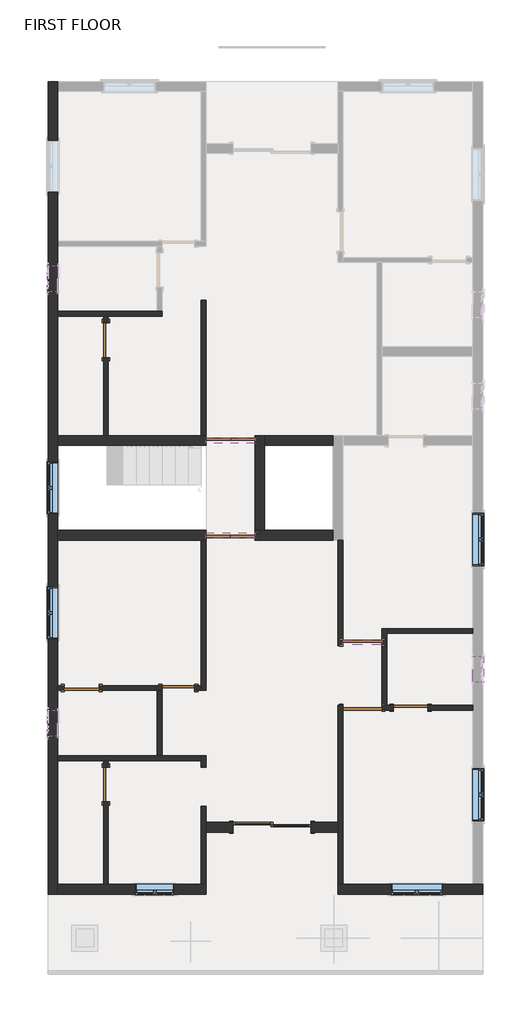
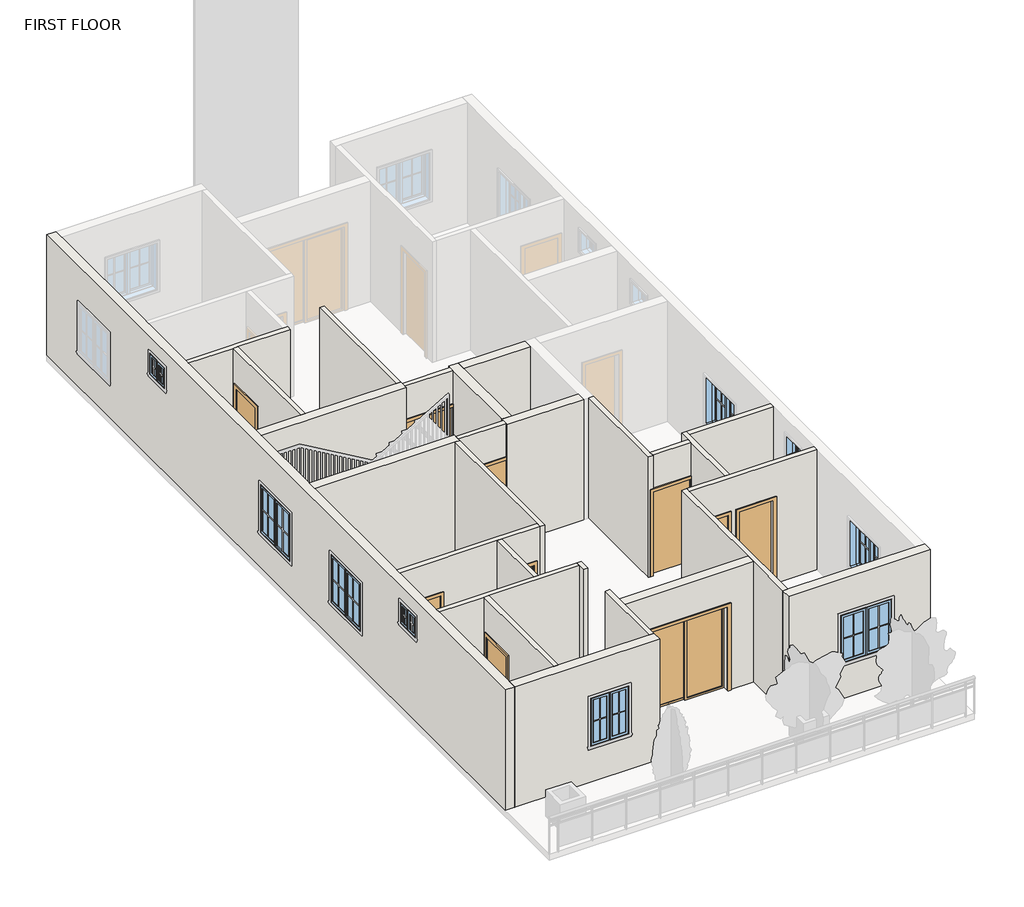
# One storey, part 1 of 4: 27 walls, 10 doors, 9 windows.
"""IFC4 building model written with IfcOpenShell, lengths in millimetres."""

from ifc_helpers import new_model, si_unit, frame, origin, place, context, project, spatial, polyline, outline, extrude, faceted_brep, transform, mapped, element, save
from components import door_31bd1cdd, door_d4d75d1e, door_214872d5, door_d141acb4, door_38851409, single_flush_3_x7_e5f9f3c4, single_flush_3_x7_305aa2a5, window_79894727, window_casement_double_3_x4_d341e8ac, window_casement_double_4_x4_af3140d2

model = new_model("IFC4")

# Units and contexts
model_context = context("Model", 3, world=origin())
ifc_project = project(units=[si_unit("LENGTHUNIT", "METRE", prefix="MILLI")], contexts=[model_context])

# Site, building, storey
site = spatial("IfcSite", under=ifc_project)
building = spatial("IfcBuilding", under=site)
storey = spatial("IfcBuildingStorey", under=building, Name="FIRST FLOOR", Elevation=3200.4)

# Doors
placement = place(None, origin())
door_shape = door_31bd1cdd(model_context)
element("IfcDoor", 1, ObjectType="Door-Double-Flush_Panel : 3'9\"X7'", at=placement, inside=storey, context=model_context, shape_type="MappedRepresentation", body=[
    mapped(door_shape, transform((-2091.0289041, 1664.1153263, 3200.4), x_axis=(1.0, 0.0, 0.0), y_axis=(0.0, 1.0, 0.0), z_axis=(0.0, 0.0, 1.0))),
])
element("IfcDoor", 2, ObjectType="Door-Double-Flush_Panel : 3'9\"X7'", at=placement, inside=storey, context=model_context, shape_type="MappedRepresentation", body=[
    mapped(door_shape, transform((-2091.0289041, -545.7007836, 3200.4), x_axis=(-1.0, 0.0, 0.0), y_axis=(0.0, -1.0, 0.0), z_axis=(0.0, 0.0, 1.0))),
])
door_2_shape = door_d4d75d1e(model_context)
element("IfcDoor", 3, ObjectType="Door-Double-Sliding : 72\" x 84\"", at=placement, inside=storey, context=model_context, shape_type="MappedRepresentation", body=[
    mapped(door_2_shape, transform((-1119.4789041, -7505.2846737, 3200.4), x_axis=(1.0, 0.0, 0.0), y_axis=(0.0, 1.0, 0.0), z_axis=(0.0, 0.0, 1.0))),
])
door_3_shape = door_214872d5(model_context)
element("IfcDoor", 4, ObjectType="Single-Flush : 2'6\"X7'", at=placement, inside=storey, context=model_context, shape_type="MappedRepresentation", body=[
    mapped(door_3_shape, transform((-3310.2289041, -4120.7346737, 3200.4), x_axis=(1.0, 0.0, 0.0), y_axis=(0.0, 1.0, 0.0), z_axis=(0.0, 0.0, 1.0))),
])
door_4_shape = door_d141acb4(model_context)
element("IfcDoor", 5, ObjectType="Single-Flush : 2'8\"X7'", at=placement, inside=storey, context=model_context, shape_type="MappedRepresentation", body=[
    mapped(door_4_shape, transform((-5005.6789041, 4013.6153263, 3200.4), x_axis=(0.0, 1.0, 0.0), y_axis=(-1.0, 0.0, 0.0), z_axis=(0.0, 0.0, 1.0))),
])
element("IfcDoor", 6, ObjectType="Single-Flush : 2'8\"X7'", at=placement, inside=storey, context=model_context, shape_type="MappedRepresentation", body=[
    mapped(door_4_shape, transform((-5570.8289041, -4120.7346737, 3200.4), x_axis=(-1.0, 0.0, 0.0), y_axis=(0.0, -1.0, 0.0), z_axis=(0.0, 0.0, 1.0))),
])
element("IfcDoor", 7, ObjectType="Single-Flush : 2'8\"X7'", at=placement, inside=storey, context=model_context, shape_type="MappedRepresentation", body=[
    mapped(door_4_shape, transform((-5005.6789041, -6374.9846737, 3200.4), x_axis=(0.0, 1.0, 0.0), y_axis=(-1.0, 0.0, 0.0), z_axis=(0.0, 0.0, 1.0))),
])
door_5_shape = door_38851409(model_context)
element("IfcDoor", 8, ObjectType="Single-Flush : 2'8\"X7'", at=placement, inside=storey, context=model_context, shape_type="MappedRepresentation", body=[
    mapped(door_5_shape, transform((2125.3710959, -4577.9346737, 3200.4), x_axis=(-1.0, 0.0, 0.0), y_axis=(0.0, -1.0, 0.0), z_axis=(0.0, 0.0, 1.0))),
])
single_flush_3_x7_shape = single_flush_3_x7_e5f9f3c4(model_context)
element("IfcDoor", 9, ObjectType="Single-Flush : 3'X7'", at=placement, inside=storey, context=model_context, shape_type="MappedRepresentation", body=[
    mapped(single_flush_3_x7_shape, transform((995.0710959, -4577.9346737, 3200.4), x_axis=(-1.0, 0.0, 0.0), y_axis=(0.0, -1.0, 0.0), z_axis=(0.0, 0.0, 1.0))),
])
single_flush_3_x7_2_shape = single_flush_3_x7_305aa2a5(model_context)
element("IfcDoor", 10, ObjectType="Single-Flush : 3'X7'", at=placement, inside=storey, context=model_context, shape_type="MappedRepresentation", body=[
    mapped(single_flush_3_x7_2_shape, transform((995.0710959, -3056.3085282, 3200.4), x_axis=(-1.0, 0.0, 0.0), y_axis=(0.0, -1.0, 0.0), z_axis=(0.0, 0.0, 1.0))),
])

# Walls
element("IfcWall", 11, ObjectType="4.5\"", at=placement, inside=storey, context=model_context, shape_type="Brep", body=[
    faceted_brep([(-6129.6289041, 4572.4153263, 3200.4), (-5062.8289041, 4572.4153263, 3200.4), (-4948.5289041, 4572.4153263, 3200.4), (-3691.2289041, 4572.4153263, 3200.4), (-3691.2289041, 4572.4153263, 6248.4), (-4948.5289041, 4572.4153263, 6248.4), (-5062.8289041, 4572.4153263, 6248.4), (-6129.6289041, 4572.4153263, 6248.4), (-6129.6289041, 4686.7153263, 3200.4), (-6129.6289041, 4686.7153263, 6248.4), (-3805.5289041, 4686.7153263, 6248.4), (-3691.2289041, 4686.7153263, 6248.4), (-3691.2289041, 4686.7153263, 3200.4), (-3805.5289041, 4686.7153263, 3200.4)], [[[0, 1, 2, 3, 4, 5, 6, 7]], [[8, 9, 10, 11, 12, 13]], [[3, 2, 1, 0, 8, 13, 12]], [[7, 6, 5, 4, 11, 10, 9]], [[0, 7, 9, 8]], [[4, 3, 12, 11]]]),
])
element("IfcWall", 12, ObjectType="4.5\"", at=placement, inside=storey, context=model_context, shape_type="SweptSolid", body=[
    extrude(outline(polyline([(4572.4153263, 3200.4), (4420.0153263, 3200.4), (4420.0153263, 5334.0), (3607.2153263, 5334.0), (3607.2153263, 3200.4), (1778.4153263, 3200.4), (1778.4153263, 6248.4), (4572.4153263, 6248.4), (4572.4153263, 3200.4)])), frame((-5062.8289041, 0.0, 0.0), z_axis=(1.0, 0.0, 0.0), x_axis=(0.0, 1.0, 0.0)), (0.0, 0.0, 1.0), 114.3),
])
element("IfcWall", 13, ObjectType="4.5\"", at=placement, inside=storey, context=model_context, shape_type="SweptSolid", body=[
    extrude(outline(polyline([(-2776.8289041, 1778.4153263), (-2776.8289041, 4948.2268555), (-2662.5289041, 4948.2268555), (-2662.5289041, 1778.4153263), (-2776.8289041, 1778.4153263)])), frame((0.0, 0.0, 3200.4), z_axis=(0.0, 0.0, 1.0), x_axis=(1.0, 0.0, 0.0)), (0.0, 0.0, 1.0), 3048.0),
])
element("IfcWall", 14, ObjectType="4.5\"", at=placement, inside=storey, context=model_context, shape_type="Brep", body=[
    faceted_brep([(-2776.8289041, -659.9846737, 3200.4), (-2776.8289041, -4063.5846737, 3200.4), (-2776.8289041, -4177.8846737, 3200.4), (-2776.8289041, -4177.8846737, 6248.4), (-2776.8289041, -4063.5846737, 6248.4), (-2776.8289041, -659.9846737, 6248.4), (-2662.5289041, -659.9846737, 3200.4), (-2662.5289041, -659.9846737, 6248.4), (-2662.5289041, -4177.8846737, 6248.4), (-2662.5289041, -4177.8846737, 3200.4)], [[[0, 1, 2, 3, 4, 5]], [[6, 7, 8, 9]], [[2, 1, 0, 6, 9]], [[5, 4, 3, 8, 7]], [[0, 5, 7, 6]], [[3, 2, 9, 8]]]),
])
element("IfcWall", 15, ObjectType="4.5\"", at=placement, inside=storey, context=model_context, shape_type="Brep", body=[
    faceted_brep([(-2776.8289041, -4063.5846737, 3200.4), (-2929.2289041, -4063.5846737, 3200.4), (-2929.2289041, -4063.5846737, 5334.0), (-3691.2289041, -4063.5846737, 5334.0), (-3691.2289041, -4063.5846737, 3200.4), (-5164.4289041, -4063.5846737, 3200.4), (-5164.4289041, -4063.5846737, 5334.0), (-5977.2289041, -4063.5846737, 5334.0), (-5977.2289041, -4063.5846737, 3200.4), (-6129.6289041, -4063.5846737, 3200.4), (-6129.6289041, -4063.5846737, 6248.4), (-2776.8289041, -4063.5846737, 6248.4), (-2929.2289041, -4177.8846737, 5334.0), (-2929.2289041, -4177.8846737, 3200.4), (-2776.8289041, -4177.8846737, 3200.4), (-2776.8289041, -4177.8846737, 6248.4), (-3691.2289041, -4177.8846737, 6248.4), (-3805.5289041, -4177.8846737, 6248.4), (-6129.6289041, -4177.8846737, 6248.4), (-6129.6289041, -4177.8846737, 3200.4), (-5977.2289041, -4177.8846737, 3200.4), (-5977.2289041, -4177.8846737, 5334.0), (-5164.4289041, -4177.8846737, 5334.0), (-5164.4289041, -4177.8846737, 3200.4), (-3805.5289041, -4177.8846737, 3200.4), (-3691.2289041, -4177.8846737, 3200.4), (-3691.2289041, -4177.8846737, 5334.0)], [[[0, 1, 2, 3, 4, 5, 6, 7, 8, 9, 10, 11]], [[12, 13, 14, 15, 16, 17, 18, 19, 20, 21, 22, 23, 24, 25, 26]], [[9, 8, 20, 19]], [[14, 13, 1, 0]], [[25, 24, 23, 5, 4]], [[11, 10, 18, 17, 16, 15]], [[0, 11, 15, 14]], [[10, 9, 19, 18]], [[21, 20, 8, 7]], [[22, 21, 7, 6]], [[23, 22, 6, 5]], [[2, 1, 13, 12]], [[3, 2, 12, 26]], [[4, 3, 26, 25]]]),
])
element("IfcWall", 16, ObjectType="4.5\"", at=placement, inside=storey, context=model_context, shape_type="Brep", body=[
    faceted_brep([(-3805.5289041, -4177.8846737, 3200.4), (-3805.5289041, -5701.8846737, 3200.4), (-3805.5289041, -5701.8846737, 6248.4), (-3805.5289041, -4177.8846737, 6248.4), (-3691.2289041, -4177.8846737, 3200.4), (-3691.2289041, -4177.8846737, 5334.0), (-3691.2289041, -4177.8846737, 6248.4), (-3691.2289041, -5701.8846737, 6248.4), (-3691.2289041, -5701.8846737, 3200.4)], [[[0, 1, 2, 3]], [[4, 5, 6, 7, 8]], [[1, 0, 4, 8]], [[3, 2, 7, 6]], [[0, 3, 6, 5, 4]], [[2, 1, 8, 7]]]),
])
element("IfcWall", 17, ObjectType="4.5\"", at=placement, inside=storey, context=model_context, shape_type="Brep", body=[
    faceted_brep([(-6129.6289041, -5816.1846737, 3200.4), (-5062.8289041, -5816.1846737, 3200.4), (-4948.5289041, -5816.1846737, 3200.4), (-2776.8289041, -5816.1846737, 3200.4), (-2776.8289041, -5816.1846737, 6248.4), (-4948.5289041, -5816.1846737, 6248.4), (-5062.8289041, -5816.1846737, 6248.4), (-6129.6289041, -5816.1846737, 6248.4), (-6129.6289041, -5701.8846737, 3200.4), (-6129.6289041, -5701.8846737, 6248.4), (-3805.5289041, -5701.8846737, 6248.4), (-3691.2289041, -5701.8846737, 6248.4), (-2776.8289041, -5701.8846737, 6248.4), (-2776.8289041, -5701.8846737, 3200.4), (-3691.2289041, -5701.8846737, 3200.4), (-3805.5289041, -5701.8846737, 3200.4)], [[[0, 1, 2, 3, 4, 5, 6, 7]], [[8, 9, 10, 11, 12, 13, 14, 15]], [[3, 2, 1, 0, 8, 15, 14, 13]], [[7, 6, 5, 4, 12, 11, 10, 9]], [[0, 7, 9, 8]], [[4, 3, 13, 12]]]),
])
element("IfcWall", 18, ObjectType="4.5\"", at=placement, inside=storey, context=model_context, shape_type="Brep", body=[
    faceted_brep([(-2776.8289041, -5701.8846737, 3200.4), (-2776.8289041, -5816.1846737, 3200.4), (-2776.8289041, -5968.5846737, 3200.4), (-2776.8289041, -5968.5846737, 6248.4), (-2776.8289041, -5816.1846737, 6248.4), (-2776.8289041, -5701.8846737, 6248.4), (-2662.5289041, -5701.8846737, 3200.4), (-2662.5289041, -5701.8846737, 6248.4), (-2662.5289041, -5968.5846737, 6248.4), (-2662.5289041, -5968.5846737, 3200.4)], [[[0, 1, 2, 3, 4, 5]], [[6, 7, 8, 9]], [[2, 1, 0, 6, 9]], [[3, 2, 9, 8]], [[5, 4, 3, 8, 7]], [[0, 5, 7, 6]]]),
])
element("IfcWall", 19, ObjectType="4.5\"", at=placement, inside=storey, context=model_context, shape_type="SweptSolid", body=[
    extrude(outline(polyline([(-5816.1846737, 3200.4), (-5968.5846737, 3200.4), (-5968.5846737, 5334.0), (-6781.3846737, 5334.0), (-6781.3846737, 3200.4), (-8711.7846737, 3200.4), (-8711.7846737, 6248.4), (-5816.1846737, 6248.4), (-5816.1846737, 3200.4)])), frame((-5062.8289041, 0.0, 0.0), z_axis=(1.0, 0.0, 0.0), x_axis=(0.0, 1.0, 0.0)), (0.0, 0.0, 1.0), 114.3),
])
element("IfcWall", 20, ObjectType="4.5\"", at=placement, inside=storey, context=model_context, shape_type="Brep", body=[
    faceted_brep([(-2776.8289041, -6882.9846737, 3200.4), (-2776.8289041, -8711.7846737, 3200.4), (-2776.8289041, -8711.7846737, 6248.4), (-2776.8289041, -6882.9846737, 6248.4), (-2662.5289041, -6882.9846737, 3200.4), (-2662.5289041, -6882.9846737, 6248.4), (-2662.5289041, -7263.9846737, 6248.4), (-2662.5289041, -7492.5846737, 6248.4), (-2662.5289041, -8711.7846737, 6248.4), (-2662.5289041, -8711.7846737, 3200.4), (-2662.5289041, -7492.5846737, 3200.4), (-2662.5289041, -7263.9846737, 3200.4)], [[[0, 1, 2, 3]], [[4, 5, 6, 7, 8, 9, 10, 11]], [[1, 0, 4, 11, 10, 9]], [[3, 2, 8, 7, 6, 5]], [[0, 3, 5, 4]], [[2, 1, 9, 8]]]),
])
element("IfcWall", 21, ObjectType="4.5\"", at=placement, inside=storey, context=model_context, shape_type="Brep", body=[
    faceted_brep([(423.5710959, -659.9846737, 3200.4), (423.5710959, -3136.3185282, 3200.4), (423.5710959, -3136.3185282, 6248.4), (423.5710959, -659.9846737, 6248.4), (537.8710959, -659.9846737, 3200.4), (537.8710959, -659.9846737, 6248.4), (537.8710959, -2999.1585282, 6248.4), (537.8710959, -3113.4585282, 6248.4), (537.8710959, -3136.3185282, 6248.4), (537.8710959, -3136.3185282, 3200.4), (537.8710959, -3113.4585282, 3200.4), (537.8710959, -2999.1585282, 3200.4)], [[[0, 1, 2, 3]], [[4, 5, 6, 7, 8, 9, 10, 11]], [[1, 0, 4, 11, 10, 9]], [[2, 1, 9, 8]], [[3, 2, 8, 7, 6, 5]], [[0, 3, 5, 4]]]),
])
element("IfcWall", 22, ObjectType="4.5\"", at=placement, inside=storey, context=model_context, shape_type="Brep", body=[
    faceted_brep([(423.5710959, -4520.7846737, 3200.4), (423.5710959, -7263.9846737, 3200.4), (423.5710959, -7492.5846737, 3200.4), (423.5710959, -8711.7846737, 3200.4), (423.5710959, -8711.7846737, 6248.4), (423.5710959, -7492.5846737, 6248.4), (423.5710959, -7263.9846737, 6248.4), (423.5710959, -4520.7846737, 6248.4), (537.8710959, -4520.7846737, 3200.4), (537.8710959, -4520.7846737, 5334.0), (537.8710959, -4520.7846737, 6248.4), (537.8710959, -4635.0846737, 6248.4), (537.8710959, -8711.7846737, 6248.4), (537.8710959, -8711.7846737, 3200.4)], [[[0, 1, 2, 3, 4, 5, 6, 7]], [[8, 9, 10, 11, 12, 13]], [[3, 2, 1, 0, 8, 13]], [[7, 6, 5, 4, 12, 11, 10]], [[4, 3, 13, 12]], [[0, 7, 10, 9, 8]]]),
])
element("IfcWall", 23, ObjectType="4.5\"", at=placement, inside=storey, context=model_context, shape_type="Brep", body=[
    faceted_brep([(1718.9710959, -4520.7846737, 5334.0), (1718.9710959, -4520.7846737, 3200.4), (1566.5710959, -4520.7846737, 3200.4), (1452.2710959, -4520.7846737, 3200.4), (1452.2710959, -4520.7846737, 5334.0), (537.8710959, -4520.7846737, 5334.0), (537.8710959, -4520.7846737, 6248.4), (1452.2710959, -4520.7846737, 6248.4), (1566.5710959, -4520.7846737, 6248.4), (3585.8710959, -4520.7846737, 6248.4), (3585.8710959, -4520.7846737, 3200.4), (2531.7710959, -4520.7846737, 3200.4), (2531.7710959, -4520.7846737, 5334.0), (1452.2710959, -4635.0846737, 3200.4), (1718.9710959, -4635.0846737, 3200.4), (1718.9710959, -4635.0846737, 5334.0), (2531.7710959, -4635.0846737, 5334.0), (2531.7710959, -4635.0846737, 3200.4), (3585.8710959, -4635.0846737, 3200.4), (3585.8710959, -4635.0846737, 6248.4), (537.8710959, -4635.0846737, 6248.4), (537.8710959, -4635.0846737, 5334.0), (1452.2710959, -4635.0846737, 5334.0)], [[[0, 1, 2, 3, 4, 5, 6, 7, 8, 9, 10, 11, 12]], [[13, 14, 15, 16, 17, 18, 19, 20, 21, 22]], [[11, 10, 18, 17]], [[3, 2, 1, 14, 13]], [[9, 8, 7, 6, 20, 19]], [[10, 9, 19, 18]], [[20, 6, 5, 21]], [[4, 22, 21, 5]], [[22, 4, 3, 13]], [[15, 14, 1, 0]], [[16, 15, 0, 12]], [[17, 16, 12, 11]]]),
])
element("IfcWall", 24, ObjectType="4.5\"", at=placement, inside=storey, context=model_context, shape_type="Brep", body=[
    faceted_brep([(1566.5710959, -4520.7846737, 3200.4), (1566.5710959, -2844.3846737, 3200.4), (1566.5710959, -2730.0846737, 3200.4), (1566.5710959, -2730.0846737, 6248.4), (1566.5710959, -2844.3846737, 6248.4), (1566.5710959, -4520.7846737, 6248.4), (1452.2710959, -4520.7846737, 3200.4), (1452.2710959, -4520.7846737, 5334.0), (1452.2710959, -4520.7846737, 6248.4), (1452.2710959, -3113.4585282, 6248.4), (1452.2710959, -2999.1585282, 6248.4), (1452.2710959, -2730.0846737, 6248.4), (1452.2710959, -2730.0846737, 3200.4), (1452.2710959, -2999.1585282, 3200.4), (1452.2710959, -3113.4585282, 3200.4)], [[[0, 1, 2, 3, 4, 5]], [[6, 7, 8, 9, 10, 11, 12, 13, 14]], [[2, 1, 0, 6, 14, 13, 12]], [[5, 4, 3, 11, 10, 9, 8]], [[0, 5, 8, 7, 6]], [[3, 2, 12, 11]]]),
])
element("IfcWall", 25, ObjectType="4.5\"", at=placement, inside=storey, context=model_context, shape_type="SweptSolid", body=[
    extrude(outline(polyline([(3585.8710959, -2844.3846737), (1566.5710959, -2844.3846737), (1566.5710959, -2730.0846737), (3585.8710959, -2730.0846737), (3585.8710959, -2844.3846737)])), frame((0.0, 0.0, 3200.4), z_axis=(0.0, 0.0, 1.0), x_axis=(1.0, 0.0, 0.0)), (0.0, 0.0, 1.0), 3048.0),
])
element("IfcWall", 26, ObjectType="4.5\"", at=placement, inside=storey, context=model_context, shape_type="SweptSolid", body=[
    extrude(outline(polyline([(-1519.5289041, 1606.9653263), (-2662.5289041, 1606.9653263), (-2662.5289041, 1721.2653263), (-1519.5289041, 1721.2653263), (-1519.5289041, 1606.9653263)])), frame((0.0, 0.0, 5334.0), z_axis=(0.0, 0.0, 1.0), x_axis=(1.0, 0.0, 0.0)), (0.0, 0.0, 1.0), 914.4),
])
element("IfcWall", 27, ObjectType="4.5\"", at=placement, inside=storey, context=model_context, shape_type="SweptSolid", body=[
    extrude(outline(polyline([(-1519.5289041, -602.8507836), (-2662.5289041, -602.8507836), (-2662.5289041, -488.5507836), (-1519.5289041, -488.5507836), (-1519.5289041, -602.8507836)])), frame((0.0, 0.0, 5334.0), z_axis=(0.0, 0.0, 1.0), x_axis=(1.0, 0.0, 0.0)), (0.0, 0.0, 1.0), 914.4),
])
element("IfcWall", 28, ObjectType="4.5\"", at=placement, inside=storey, context=model_context, shape_type="SweptSolid", body=[
    extrude(outline(polyline([(1452.2710959, -3113.4585282), (537.8710959, -3113.4585282), (537.8710959, -2999.1585282), (1452.2710959, -2999.1585282), (1452.2710959, -3113.4585282)])), frame((0.0, 0.0, 5334.0), z_axis=(0.0, 0.0, 1.0), x_axis=(1.0, 0.0, 0.0)), (0.0, 0.0, 1.0), 914.4),
])
element("IfcWall", 29, ObjectType="9\"", at=placement, inside=storey, context=model_context, shape_type="Brep", body=[
    faceted_brep([(-6358.2289041, 10058.8153263, 3200.4), (-6358.2289041, -8940.3846737, 3200.4), (-6358.2289041, -8940.3846737, 6248.4), (-6358.2289041, 10058.8153263, 6248.4), (-6358.2289041, 8687.2153263, 5334.0), (-6358.2289041, 7468.0153263, 5334.0), (-6358.2289041, 7468.0153263, 4114.8), (-6358.2289041, 8687.2153263, 4114.8), (-6358.2289041, -1752.1846737, 5334.0), (-6358.2289041, -2971.3846737, 5334.0), (-6358.2289041, -2971.3846737, 4114.8), (-6358.2289041, -1752.1846737, 4114.8), (-6358.2289041, 1168.8153263, 5334.0), (-6358.2289041, -50.3846737, 5334.0), (-6358.2289041, -50.3846737, 4114.8), (-6358.2289041, 1168.8153263, 4114.8), (-6358.2289041, 5753.5153263, 5867.4), (-6358.2289041, 5143.9153263, 5867.4), (-6358.2289041, 5143.9153263, 5334.0), (-6358.2289041, 5753.5153263, 5334.0), (-6358.2289041, -4635.0846737, 5867.4), (-6358.2289041, -5244.6846737, 5867.4), (-6358.2289041, -5244.6846737, 5334.0), (-6358.2289041, -4635.0846737, 5334.0), (-6129.6289041, 10058.8153263, 3200.4), (-6129.6289041, 10058.8153263, 6248.4), (-6129.6289041, 9830.2153263, 6248.4), (-6129.6289041, 6325.0153263, 6248.4), (-6129.6289041, 6210.7153263, 6248.4), (-6129.6289041, 4686.7153263, 6248.4), (-6129.6289041, 4572.4153263, 6248.4), (-6129.6289041, 1778.4153263, 6248.4), (-6129.6289041, 1549.8153263, 6248.4), (-6129.6289041, -431.3846737, 6248.4), (-6129.6289041, -659.9846737, 6248.4), (-6129.6289041, -4063.5846737, 6248.4), (-6129.6289041, -4177.8846737, 6248.4), (-6129.6289041, -5701.8846737, 6248.4), (-6129.6289041, -5816.1846737, 6248.4), (-6129.6289041, -8711.7846737, 6248.4), (-6129.6289041, -8940.3846737, 6248.4), (-6129.6289041, -8940.3846737, 3200.4), (-6129.6289041, -8711.7846737, 3200.4), (-6129.6289041, -5816.1846737, 3200.4), (-6129.6289041, -5701.8846737, 3200.4), (-6129.6289041, -4177.8846737, 3200.4), (-6129.6289041, -4063.5846737, 3200.4), (-6129.6289041, -659.9846737, 3200.4), (-6129.6289041, -431.3846737, 3200.4), (-6129.6289041, 1549.8153263, 3200.4), (-6129.6289041, 1778.4153263, 3200.4), (-6129.6289041, 4572.4153263, 3200.4), (-6129.6289041, 4686.7153263, 3200.4), (-6129.6289041, 6210.7153263, 3200.4), (-6129.6289041, 6325.0153263, 3200.4), (-6129.6289041, 9830.2153263, 3200.4), (-6129.6289041, 8687.2153263, 5334.0), (-6129.6289041, 8687.2153263, 4114.8), (-6129.6289041, 7468.0153263, 4114.8), (-6129.6289041, 7468.0153263, 5334.0), (-6129.6289041, -1752.1846737, 5334.0), (-6129.6289041, -1752.1846737, 4114.8), (-6129.6289041, -2971.3846737, 4114.8), (-6129.6289041, -2971.3846737, 5334.0), (-6129.6289041, 1168.8153263, 5334.0), (-6129.6289041, 1168.8153263, 4114.8), (-6129.6289041, -50.3846737, 4114.8), (-6129.6289041, -50.3846737, 5334.0), (-6129.6289041, 5753.5153263, 5867.4), (-6129.6289041, 5753.5153263, 5334.0), (-6129.6289041, 5143.9153263, 5334.0), (-6129.6289041, 5143.9153263, 5867.4), (-6129.6289041, -4635.0846737, 5867.4), (-6129.6289041, -4635.0846737, 5334.0), (-6129.6289041, -5244.6846737, 5334.0), (-6129.6289041, -5244.6846737, 5867.4)], [[[0, 1, 2, 3], [4, 5, 6, 7], [8, 9, 10, 11], [12, 13, 14, 15], [16, 17, 18, 19], [20, 21, 22, 23]], [[24, 25, 26, 27, 28, 29, 30, 31, 32, 33, 34, 35, 36, 37, 38, 39, 40, 41, 42, 43, 44, 45, 46, 47, 48, 49, 50, 51, 52, 53, 54, 55], [56, 57, 58, 59], [60, 61, 62, 63], [64, 65, 66, 67], [68, 69, 70, 71], [72, 73, 74, 75]], [[1, 0, 24, 55, 54, 53, 52, 51, 50, 49, 48, 47, 46, 45, 44, 43, 42, 41]], [[3, 2, 40, 39, 38, 37, 36, 35, 34, 33, 32, 31, 30, 29, 28, 27, 26, 25]], [[2, 1, 41, 40]], [[0, 3, 25, 24]], [[57, 56, 4, 7]], [[58, 57, 7, 6]], [[59, 58, 6, 5]], [[56, 59, 5, 4]], [[61, 60, 8, 11]], [[62, 61, 11, 10]], [[63, 62, 10, 9]], [[60, 63, 9, 8]], [[65, 64, 12, 15]], [[66, 65, 15, 14]], [[67, 66, 14, 13]], [[64, 67, 13, 12]], [[69, 68, 16, 19]], [[70, 69, 19, 18]], [[71, 70, 18, 17]], [[68, 71, 17, 16]], [[73, 72, 20, 23]], [[74, 73, 23, 22]], [[75, 74, 22, 21]], [[72, 75, 21, 20]]]),
])
element("IfcWall", 30, ObjectType="9\"", at=placement, inside=storey, context=model_context, shape_type="Brep", body=[
    faceted_brep([(-6129.6289041, -8940.3846737, 3200.4), (-2662.5289041, -8940.3846737, 3200.4), (-2662.5289041, -8940.3846737, 6248.4), (-6129.6289041, -8940.3846737, 6248.4), (-4319.8789041, -8940.3846737, 5334.0), (-3405.4789041, -8940.3846737, 5334.0), (-3405.4789041, -8940.3846737, 4114.8), (-4319.8789041, -8940.3846737, 4114.8), (-6129.6289041, -8711.7846737, 3200.4), (-6129.6289041, -8711.7846737, 6248.4), (-5062.8289041, -8711.7846737, 6248.4), (-4948.5289041, -8711.7846737, 6248.4), (-2776.8289041, -8711.7846737, 6248.4), (-2662.5289041, -8711.7846737, 6248.4), (-2662.5289041, -8711.7846737, 3200.4), (-2776.8289041, -8711.7846737, 3200.4), (-4948.5289041, -8711.7846737, 3200.4), (-5062.8289041, -8711.7846737, 3200.4), (-4319.8789041, -8711.7846737, 5334.0), (-4319.8789041, -8711.7846737, 4114.8), (-3405.4789041, -8711.7846737, 4114.8), (-3405.4789041, -8711.7846737, 5334.0)], [[[0, 1, 2, 3], [4, 5, 6, 7]], [[8, 9, 10, 11, 12, 13, 14, 15, 16, 17], [18, 19, 20, 21]], [[1, 0, 8, 17, 16, 15, 14]], [[3, 2, 13, 12, 11, 10, 9]], [[0, 3, 9, 8]], [[2, 1, 14, 13]], [[19, 18, 4, 7]], [[20, 19, 7, 6]], [[21, 20, 6, 5]], [[18, 21, 5, 4]]]),
])
element("IfcWall", 31, ObjectType="9\"", at=placement, inside=storey, context=model_context, shape_type="Brep", body=[
    faceted_brep([(423.5710959, -8940.3846737, 3200.4), (3814.4710959, -8940.3846737, 3200.4), (3814.4710959, -8940.3846737, 6248.4), (423.5710959, -8940.3846737, 6248.4), (1662.2107801, -8940.3846737, 5334.0), (2881.4107801, -8940.3846737, 5334.0), (2881.4107801, -8940.3846737, 4114.8), (1662.2107801, -8940.3846737, 4114.8), (423.5710959, -8711.7846737, 3200.4), (423.5710959, -8711.7846737, 6248.4), (537.8710959, -8711.7846737, 6248.4), (3585.8710959, -8711.7846737, 6248.4), (3814.4710959, -8711.7846737, 6248.4), (3814.4710959, -8711.7846737, 3200.4), (3585.8710959, -8711.7846737, 3200.4), (537.8710959, -8711.7846737, 3200.4), (1662.2107801, -8711.7846737, 5334.0), (1662.2107801, -8711.7846737, 4114.8), (2881.4107801, -8711.7846737, 4114.8), (2881.4107801, -8711.7846737, 5334.0)], [[[0, 1, 2, 3], [4, 5, 6, 7]], [[8, 9, 10, 11, 12, 13, 14, 15], [16, 17, 18, 19]], [[1, 0, 8, 15, 14, 13]], [[3, 2, 12, 11, 10, 9]], [[2, 1, 13, 12]], [[0, 3, 9, 8]], [[17, 16, 4, 7]], [[18, 17, 7, 6]], [[19, 18, 6, 5]], [[16, 19, 5, 4]]]),
])
element("IfcWall", 32, ObjectType="9\"", at=placement, inside=storey, context=model_context, shape_type="Brep", body=[
    faceted_brep([(-6129.6289041, 1549.8153263, 3200.4), (-2662.5289041, 1549.8153263, 3200.4), (-2662.5289041, 1549.8153263, 6248.4), (-6129.6289041, 1549.8153263, 6248.4), (-6129.6289041, 1778.4153263, 3200.4), (-6129.6289041, 1778.4153263, 6248.4), (-5062.8289041, 1778.4153263, 6248.4), (-4948.5289041, 1778.4153263, 6248.4), (-2776.8289041, 1778.4153263, 6248.4), (-2662.5289041, 1778.4153263, 6248.4), (-2662.5289041, 1778.4153263, 3200.4), (-2776.8289041, 1778.4153263, 3200.4), (-4948.5289041, 1778.4153263, 3200.4), (-5062.8289041, 1778.4153263, 3200.4), (-2662.5289041, 1606.9653263, 6248.4), (-2662.5289041, 1721.2653263, 6248.4)], [[[0, 1, 2, 3]], [[4, 5, 6, 7, 8, 9, 10, 11, 12, 13]], [[1, 0, 4, 13, 12, 11, 10]], [[3, 2, 14, 15, 9, 8, 7, 6, 5]], [[0, 3, 5, 4]], [[2, 1, 10, 9, 15, 14]]]),
])
element("IfcWall", 33, ObjectType="9\"", at=placement, inside=storey, context=model_context, shape_type="Brep", body=[
    faceted_brep([(-6129.6289041, -659.9846737, 3200.4), (-2776.8289041, -659.9846737, 3200.4), (-2662.5289041, -659.9846737, 3200.4), (-2662.5289041, -659.9846737, 6248.4), (-2776.8289041, -659.9846737, 6248.4), (-6129.6289041, -659.9846737, 6248.4), (-6129.6289041, -431.3846737, 3200.4), (-6129.6289041, -431.3846737, 6248.4), (-2662.5289041, -431.3846737, 6248.4), (-2662.5289041, -431.3846737, 3200.4), (-2662.5289041, -602.8507836, 6248.4), (-2662.5289041, -488.5507836, 6248.4)], [[[0, 1, 2, 3, 4, 5]], [[6, 7, 8, 9]], [[2, 1, 0, 6, 9]], [[5, 4, 3, 10, 11, 8, 7]], [[0, 5, 7, 6]], [[3, 2, 9, 8, 11, 10]]]),
])
element("IfcWall", 34, ObjectType="9\"", at=placement, inside=storey, context=model_context, shape_type="Brep", body=[
    faceted_brep([(309.2710959, -431.3846737, 3200.4), (-1290.9289041, -431.3846737, 3200.4), (-1519.5289041, -431.3846737, 3200.4), (-1519.5289041, -431.3846737, 6248.4), (-1290.9289041, -431.3846737, 6248.4), (309.2710959, -431.3846737, 6248.4), (309.2710959, -659.9846737, 3200.4), (309.2710959, -659.9846737, 6248.4), (-1519.5289041, -659.9846737, 6248.4), (-1519.5289041, -659.9846737, 3200.4), (-1519.5289041, -488.5507836, 6248.4), (-1519.5289041, -602.8507836, 6248.4)], [[[0, 1, 2, 3, 4, 5]], [[6, 7, 8, 9]], [[2, 1, 0, 6, 9]], [[5, 4, 3, 10, 11, 8, 7]], [[0, 5, 7, 6]], [[3, 2, 9, 8, 11, 10]]]),
])
element("IfcWall", 35, ObjectType="9\"", at=placement, inside=storey, context=model_context, shape_type="Brep", body=[
    faceted_brep([(-1290.9289041, -431.3846737, 3200.4), (-1290.9289041, 1549.8153263, 3200.4), (-1290.9289041, 1778.4153263, 3200.4), (-1290.9289041, 1778.4153263, 6248.4), (-1290.9289041, 1549.8153263, 6248.4), (-1290.9289041, -431.3846737, 6248.4), (-1519.5289041, -431.3846737, 3200.4), (-1519.5289041, -431.3846737, 6248.4), (-1519.5289041, 1606.9653263, 6248.4), (-1519.5289041, 1721.2653263, 6248.4), (-1519.5289041, 1778.4153263, 6248.4), (-1519.5289041, 1778.4153263, 3200.4)], [[[0, 1, 2, 3, 4, 5]], [[6, 7, 8, 9, 10, 11]], [[2, 1, 0, 6, 11]], [[5, 4, 3, 10, 9, 8, 7]], [[0, 5, 7, 6]], [[3, 2, 11, 10]]]),
])
element("IfcWall", 36, ObjectType="9\"", at=placement, inside=storey, context=model_context, shape_type="SweptSolid", body=[
    extrude(outline(polyline([(-1290.9289041, 1778.4153263), (309.2710959, 1778.4153263), (309.2710959, 1549.8153263), (-1290.9289041, 1549.8153263), (-1290.9289041, 1778.4153263)])), frame((0.0, 0.0, 3200.4), z_axis=(0.0, 0.0, 1.0), x_axis=(1.0, 0.0, 0.0)), (0.0, 0.0, 1.0), 3048.0),
])
element("IfcWall", 37, ObjectType="9\"", at=placement, inside=storey, context=model_context, shape_type="SweptSolid", body=[
    extrude(outline(polyline([(5334.0, -205.0789041), (3200.4, -205.0789041), (3200.4, 423.5710959), (6248.4, 423.5710959), (6248.4, -2662.5289041), (3200.4, -2662.5289041), (3200.4, -2033.8789041), (5334.0, -2033.8789041), (5334.0, -205.0789041)])), frame((0.0, -7492.5846737, 0.0), z_axis=(0.0, 1.0, 0.0), x_axis=(0.0, 0.0, 1.0)), (0.0, 0.0, 1.0), 228.6),
])

# Windows
window_shape = window_79894727(model_context)
element("IfcWindow", 38, ObjectType="Window-Casement-Double : 2'X1'9\"", at=placement, inside=storey, context=model_context, shape_type="MappedRepresentation", body=[
    mapped(window_shape, transform((-6243.9289041, 5448.7153263, 3200.4), x_axis=(0.0, 1.0, 0.0), y_axis=(-1.0, 0.0, 0.0), z_axis=(0.0, 0.0, 1.0))),
])
element("IfcWindow", 39, ObjectType="Window-Casement-Double : 2'X1'9\"", at=placement, inside=storey, context=model_context, shape_type="MappedRepresentation", body=[
    mapped(window_shape, transform((-6243.9289041, -4939.8846737, 3200.4), x_axis=(0.0, 1.0, 0.0), y_axis=(-1.0, 0.0, 0.0), z_axis=(0.0, 0.0, 1.0))),
])
element("IfcWindow", 40, ObjectType="Window-Casement-Double : 2'X1'9\"", at=placement, inside=storey, context=model_context, shape_type="MappedRepresentation", body=[
    mapped(window_shape, transform((3700.1710959, -3682.5846737, 3200.4), x_axis=(0.0, -1.0, 0.0), y_axis=(1.0, 0.0, 0.0), z_axis=(0.0, 0.0, 1.0))),
])
window_casement_double_3_x4_shape = window_casement_double_3_x4_d341e8ac(model_context)
element("IfcWindow", 41, ObjectType="Window-Casement-Double : 3'X4'", at=placement, inside=storey, context=model_context, shape_type="MappedRepresentation", body=[
    mapped(window_casement_double_3_x4_shape, transform((-3862.6789041, -8826.0846737, 3200.4), x_axis=(-1.0, 0.0, 0.0), y_axis=(0.0, -1.0, 0.0), z_axis=(0.0, 0.0, 1.0))),
])
window_casement_double_4_x4_shape = window_casement_double_4_x4_af3140d2(model_context)
element("IfcWindow", 42, ObjectType="Window-Casement-Double : 4'X4'", at=placement, inside=storey, context=model_context, shape_type="MappedRepresentation", body=[
    mapped(window_casement_double_4_x4_shape, transform((-6243.9289041, -2361.7846737, 3200.4), x_axis=(0.0, 1.0, 0.0), y_axis=(-1.0, 0.0, 0.0), z_axis=(0.0, 0.0, 1.0))),
])
element("IfcWindow", 43, ObjectType="Window-Casement-Double : 4'X4'", at=placement, inside=storey, context=model_context, shape_type="MappedRepresentation", body=[
    mapped(window_casement_double_4_x4_shape, transform((2271.8107801, -8826.0846737, 3200.4), x_axis=(-1.0, 0.0, 0.0), y_axis=(0.0, -1.0, 0.0), z_axis=(0.0, 0.0, 1.0))),
])
element("IfcWindow", 44, ObjectType="Window-Casement-Double : 4'X4'", at=placement, inside=storey, context=model_context, shape_type="MappedRepresentation", body=[
    mapped(window_casement_double_4_x4_shape, transform((3700.1710959, -6616.2846737, 3200.4), x_axis=(0.0, -1.0, 0.0), y_axis=(1.0, 0.0, 0.0), z_axis=(0.0, 0.0, 1.0))),
])
element("IfcWindow", 45, ObjectType="Window-Casement-Double : 4'X4'", at=placement, inside=storey, context=model_context, shape_type="MappedRepresentation", body=[
    mapped(window_casement_double_4_x4_shape, transform((3700.1710959, -647.2846737, 3200.4), x_axis=(0.0, -1.0, 0.0), y_axis=(1.0, 0.0, 0.0), z_axis=(0.0, 0.0, 1.0))),
])
element("IfcWindow", 46, ObjectType="Window-Casement-Double : 4'X4'", at=placement, inside=storey, context=model_context, shape_type="MappedRepresentation", body=[
    mapped(window_casement_double_4_x4_shape, transform((-6243.9289041, 559.2153263, 3200.4), x_axis=(0.0, 1.0, 0.0), y_axis=(-1.0, 0.0, 0.0), z_axis=(0.0, 0.0, 1.0))),
])

save(model, "model.ifc")

# Revit data of these elements
# Type "Door-Double-Flush_Panel : 3'9\"X7'"
#   Type Mark = "11"
#   Construction Type Id = "DOOR"
#   Assembly Code = "C1020"
#   Analytic Construction = "Wooden"
#   Thickness = 0' - 2"
#   Thermal Resistance (R) = 2.5876 (h·ft²·°F)/BTU
#   Swing Angle [instance default] = 90.00°
#   Panel Width = 1' - 10 1/2"
#   Heat Transfer Coefficient (U) = 0.3865 BTU/(h·ft²·°F)
#   Height = 7' - 0"
#   Trim Projection Ext = 0' - 1"
#   Trim Projection Int = 0' - 1"
#   Trim Width = 0' - 3"
#   Width = 3' - 9"
#   Define Thermal Properties by = 1
#   Panel Material = Wood - Birch - Solid Stained Light Low Gloss
#   Trim Material = Paint - Sienna
#   Visual Light Transmittance = 0
#   Solar Heat Gain Coefficient = 0
#   Function = (empty or 0)
#   Wall Closure = (empty or 0)
# Type "Door-Double-Sliding : 72\" x 84\""
#   Type Mark = "14"
#   Construction Type Id = "opn-d45"
#   Assembly Code = "C1020"
#   Analytic Construction = "Wood frame, double glass door "
#   Thickness = 0' - 2"
#   Thermal Resistance (R) = 1.8150 (h·ft²·°F)/BTU
#   Heat Transfer Coefficient (U) = 0.5510 BTU/(h·ft²·°F)
#   Height = 7' - 0"
#   Rail Width = 0' - 2"
#   Stiles = 0' - 2"
#   Trim Projection Ext = 0' - 1"
#   Trim Projection Int = 0' - 1"
#   Trim Width = 0' - 3"
#   Width = 6' - 0"
#   Define Thermal Properties by = 1
#   Glazing = Glass
#   Panel Material = Wood - Birch - Solid Stained Light Low Gloss
#   Trim Material = Paint - Sienna
#   Visual Light Transmittance = 0
#   Solar Heat Gain Coefficient = 0
#   Function = (empty or 0)
#   Wall Closure = (empty or 0)
# Type "Single-Flush : 2'6\"X7'"
#   Type Mark = "13"
#   Construction Type Id = "MDOOR"
#   Assembly Code = "C1020"
#   Analytic Construction = "Metal"
#   Thickness = 0' - 2"
#   Heat Transfer Coefficient (U) = 0.651978 BTU/(h·ft²·°F)
#   Height = 7' - 0"
#   Trim Projection Ext = 0' - 1"
#   Trim Projection Int = 0' - 1"
#   Trim Width = 0' - 3"
#   Width = 2' - 6"
#   Define Thermal Properties by = 1
#   Door Material = Door - Panel
#   Frame Material = Door - Frame
#   Visual Light Transmittance = 0
#   Solar Heat Gain Coefficient = 0
#   Function = (empty or 0)
#   Wall Closure = (empty or 0)
# Type "Single-Flush : 2'8\"X7'"
#   Type Mark = "12"
#   Construction Type Id = "MDOOR"
#   Assembly Code = "C1020"
#   Analytic Construction = "Metal"
#   Thickness = 0' - 2"
#   Heat Transfer Coefficient (U) = 0.651978 BTU/(h·ft²·°F)
#   Height = 7' - 0"
#   Trim Projection Ext = 0' - 1"
#   Trim Projection Int = 0' - 1"
#   Trim Width = 0' - 3"
#   Width = 2' - 8"
#   Define Thermal Properties by = 1
#   Door Material = Door - Panel
#   Frame Material = Door - Frame
#   Visual Light Transmittance = 0
#   Solar Heat Gain Coefficient = 0
#   Function = (empty or 0)
#   Wall Closure = (empty or 0)
# Type "Single-Flush : 3'X7'"
#   Type Mark = "8"
#   Construction Type Id = "MDOOR"
#   Assembly Code = "C1020"
#   Analytic Construction = "Metal"
#   Thickness = 0' - 2"
#   Heat Transfer Coefficient (U) = 0.651978 BTU/(h·ft²·°F)
#   Height = 7' - 0"
#   Trim Projection Ext = 0' - 1"
#   Trim Projection Int = 0' - 1"
#   Trim Width = 0' - 3"
#   Width = 3' - 0"
#   Define Thermal Properties by = 1
#   Door Material = Door - Panel
#   Frame Material = Door - Frame
#   Visual Light Transmittance = 0
#   Solar Heat Gain Coefficient = 0
#   Function = (empty or 0)
#   Wall Closure = (empty or 0)
# Type "4.5\""
#   Assembly Code = "B2010"
#   Layers, outside or top first: 0' - 4 1/2" no material (function 1)
# Type "9\""
#   Assembly Code = "B2010"
#   Layers, outside or top first: 0' - 9" "WALL" (function 1)
# Type "Window-Casement-Double : 2'X1'9\""
#   Type Mark = "22"
#   Fire Rating = "0.5h"
#   Assembly Code = "B2020100"
#   Analytic Construction = "Double glazing - domestic"
#   Frame Extension [instance default] = 0' - 0 1/4"
#   Window Inset [instance default] = 0' - 0"
#   Wall Thickness [instance default] = 0' - 6"
#   Interior Wall Closure [instance default] = 0' - 2 1/4"
#   Half Width = 1' - 0"
#   Visual Light Transmittance = 0.81
#   Thermal Resistance (R) = 1.8146 (h·ft²·°F)/BTU
#   Solar Heat Gain Coefficient = 0.76
#   Rough Width = 2' - 0 1/2"
#   Rough Height = 1' - 9 1/2"
#   Height = 1' - 9"
#   Heat Transfer Coefficient (U) = 0.5511 BTU/(h·ft²·°F)
#   Exterior Wall Closure [instance default] = 0' - 1 1/4"
#   Extension Jamb [instance default] = 0' - 2 1/4"
#   Default Sill Height = 7' - 0"
#   Width = 2' - 0"
#   Muntin Visibility = yes
#   Interior Trim Visibility [instance default] = yes
#   Exterior Trim Visibility [instance default] = yes
#   Extension Jamb Visibility [instance default] = yes
#   Interior Trim Material = Wood - Stained
#   Muntin Pattern = Muntin Pattern_2x2 : Muntin Pattern_2x2
#   Interior Trim = Trim-Window-Interior-Flat : Picture Frame
#   Interior Frame Material = Wood - Stained
#   Glass Panel Material = Glass
#   Exterior Trim Material = Clad - White
#   Exterior Trim = Trim-Window-Exterior-Flat : with Sill
#   Exterior Frame Material = Clad - White
#   Wall Closure = (empty or 0)
# Type "Window-Casement-Double : 3'X4'"
#   Type Mark = "21"
#   Fire Rating = "0.5h"
#   Assembly Code = "B2020100"
#   Analytic Construction = "Double glazing - domestic"
#   Frame Extension [instance default] = 0' - 0 1/4"
#   Window Inset [instance default] = 0' - 0"
#   Wall Thickness [instance default] = 0' - 6"
#   Interior Wall Closure [instance default] = 0' - 2 1/4"
#   Half Width = 1' - 6"
#   Visual Light Transmittance = 0.81
#   Thermal Resistance (R) = 1.8146 (h·ft²·°F)/BTU
#   Solar Heat Gain Coefficient = 0.76
#   Rough Width = 3' - 0 1/2"
#   Rough Height = 4' - 0 1/2"
#   Height = 4' - 0"
#   Heat Transfer Coefficient (U) = 0.5511 BTU/(h·ft²·°F)
#   Exterior Wall Closure [instance default] = 0' - 1 1/4"
#   Extension Jamb [instance default] = 0' - 2 1/4"
#   Default Sill Height = 3' - 0"
#   Width = 3' - 0"
#   Muntin Visibility = yes
#   Interior Trim Visibility [instance default] = yes
#   Exterior Trim Visibility [instance default] = yes
#   Extension Jamb Visibility [instance default] = yes
#   Interior Trim Material = Wood - Stained
#   Muntin Pattern = Muntin Pattern_2x2 : Muntin Pattern_2x2
#   Interior Trim = Trim-Window-Interior-Flat : Picture Frame
#   Interior Frame Material = Wood - Stained
#   Glass Panel Material = Glass
#   Exterior Trim Material = Clad - White
#   Exterior Trim = Trim-Window-Exterior-Flat : with Sill
#   Exterior Frame Material = Clad - White
#   Wall Closure = (empty or 0)
# Type "Window-Casement-Double : 4'X4'"
#   Type Mark = "20"
#   Fire Rating = "0.5h"
#   Assembly Code = "B2020100"
#   Analytic Construction = "Double glazing - domestic"
#   Frame Extension [instance default] = 0' - 0 1/4"
#   Window Inset [instance default] = 0' - 0"
#   Wall Thickness [instance default] = 0' - 6"
#   Interior Wall Closure [instance default] = 0' - 2 1/4"
#   Half Width = 2' - 0"
#   Visual Light Transmittance = 0.81
#   Thermal Resistance (R) = 1.8146 (h·ft²·°F)/BTU
#   Solar Heat Gain Coefficient = 0.76
#   Rough Width = 4' - 0 1/2"
#   Rough Height = 4' - 0 1/2"
#   Height = 4' - 0"
#   Heat Transfer Coefficient (U) = 0.5511 BTU/(h·ft²·°F)
#   Exterior Wall Closure [instance default] = 0' - 1 1/4"
#   Extension Jamb [instance default] = 0' - 2 1/4"
#   Default Sill Height = 3' - 0"
#   Width = 4' - 0"
#   Muntin Visibility = yes
#   Interior Trim Visibility [instance default] = yes
#   Exterior Trim Visibility [instance default] = yes
#   Extension Jamb Visibility [instance default] = yes
#   Interior Trim Material = Wood - Stained
#   Muntin Pattern = Muntin Pattern_2x2 : Muntin Pattern_2x2
#   Interior Trim = Trim-Window-Interior-Flat : Picture Frame
#   Interior Frame Material = Wood - Stained
#   Glass Panel Material = Glass
#   Exterior Trim Material = Clad - White
#   Exterior Trim = Trim-Window-Exterior-Flat : with Sill
#   Exterior Frame Material = Clad - White
#   Wall Closure = (empty or 0)
# Elements 1, 2 (IfcDoor, "Door-Double-Flush_Panel : 3'9\"X7'")
#   Swing Angle = 90.00°
#   Phase Created = New Construction
#   Materials on its faces: "Paint - Sienna", "Wood - Birch - Solid Stained Light Low Gloss"
# Element 3 (IfcDoor, "Door-Double-Sliding : 72\" x 84\"")
#   Phase Created = New Construction
#   Materials on its faces: "Paint - Sienna", "Wood - Birch - Solid Stained Light Low Gloss", "Glass"
# Element 4 (IfcDoor, "Single-Flush : 2'6\"X7'")
#   Phase Created = New Construction
#   Materials on its faces: "Door - Frame", "Door - Panel"
# Elements 5, 6, 7, 8 (IfcDoor, "Single-Flush : 2'8\"X7'")
#   Phase Created = New Construction
#   Materials on its faces: "Door - Frame", "Door - Panel"
# Elements 9, 10 (IfcDoor, "Single-Flush : 3'X7'")
#   Phase Created = New Construction
#   Materials on its faces: "Door - Frame", "Door - Panel"
# Elements 11, 12, 13, 14, 15, 16, 17, 18, 19, 20, 21, 22, 23, 24, 25, 26, 27, 28 (IfcWall, "4.5\"")
#   Top Offset = -0' - 6"
#   Base Offset = 0' - 0"
#   wall height = 10' - 0"
#   Phase Created = New Construction
#   Base Constraint = FIRST FLOOR
#   Top Constraint = SECOND FLOOR
#   Materials on its faces: "Default Wall"
# Element 29 (IfcWall, "9\"")
#   Top Offset = -0' - 6"
#   Base Offset = 0' - 0"
#   wall height = 10' - 0"
#   Phase Created = New Construction
#   Base Constraint = FIRST FLOOR
#   Top Constraint = SECOND FLOOR
#   Materials on its faces: "WALL", "6\" WALL"
# Element 30 (IfcWall, "9\"")
#   Top Offset = -0' - 6"
#   Base Offset = 0' - 0"
#   wall height = 10' - 0"
#   Phase Created = New Construction
#   Base Constraint = FIRST FLOOR
#   Top Constraint = SECOND FLOOR
#   Materials on its faces: "WALL", "6\" WALL", "Default Wall"
# Elements 31, 32, 33 (IfcWall, "9\"")
#   Top Offset = -0' - 6"
#   Base Offset = 0' - 0"
#   wall height = 10' - 0"
#   Phase Created = New Construction
#   Base Constraint = FIRST FLOOR
#   Top Constraint = SECOND FLOOR
#   Materials on its faces: "WALL", "Default Wall"
# Elements 34, 35, 36, 37 (IfcWall, "9\"")
#   Top Offset = -0' - 6"
#   Base Offset = 0' - 0"
#   wall height = 10' - 0"
#   Phase Created = New Construction
#   Base Constraint = FIRST FLOOR
#   Top Constraint = SECOND FLOOR
#   Materials on its faces: "WALL"
# Element 38 (IfcWindow, "Window-Casement-Double : 2'X1'9\"")
#   Mark = "26"
#   Window Inset = 0' - 0"
#   Interior Wall Closure = 0' - 2 1/4"
#   Frame Extension = 0' - 0 1/4"
#   Exterior Wall Closure = 0' - 1 1/4"
#   Interior Trim Visibility = yes
#   Exterior Trim Visibility = yes
#   Phase Created = New Construction
#   Materials on its faces: "Wood - Stained", "Glass", "Clad - White"
# Element 39 (IfcWindow, "Window-Casement-Double : 2'X1'9\"")
#   Mark = "27"
#   Window Inset = 0' - 0"
#   Interior Wall Closure = 0' - 2 1/4"
#   Frame Extension = 0' - 0 1/4"
#   Exterior Wall Closure = 0' - 1 1/4"
#   Interior Trim Visibility = yes
#   Exterior Trim Visibility = yes
#   Phase Created = New Construction
#   Materials on its faces: "Wood - Stained", "Glass", "Clad - White"
# Element 40 (IfcWindow, "Window-Casement-Double : 2'X1'9\"")
#   Mark = "28"
#   Window Inset = 0' - 0"
#   Interior Wall Closure = 0' - 2 1/4"
#   Frame Extension = 0' - 0 1/4"
#   Exterior Wall Closure = 0' - 1 1/4"
#   Interior Trim Visibility = yes
#   Exterior Trim Visibility = yes
#   Phase Created = New Construction
#   Materials on its faces: "Wood - Stained", "Glass", "Clad - White"
# Element 41 (IfcWindow, "Window-Casement-Double : 3'X4'")
#   Mark = "24"
#   Window Inset = 0' - 0"
#   Interior Wall Closure = 0' - 2 1/4"
#   Frame Extension = 0' - 0 1/4"
#   Exterior Wall Closure = 0' - 1 1/4"
#   Interior Trim Visibility = yes
#   Exterior Trim Visibility = yes
#   Phase Created = New Construction
#   Materials on its faces: "Wood - Stained", "Glass", "Clad - White"
# Element 42 (IfcWindow, "Window-Casement-Double : 4'X4'")
#   Mark = "18"
#   Window Inset = 0' - 0"
#   Interior Wall Closure = 0' - 2 1/4"
#   Frame Extension = 0' - 0 1/4"
#   Exterior Wall Closure = 0' - 1 1/4"
#   Interior Trim Visibility = yes
#   Exterior Trim Visibility = yes
#   Phase Created = New Construction
#   Materials on its faces: "Wood - Stained", "Glass", "Clad - White"
# Element 43 (IfcWindow, "Window-Casement-Double : 4'X4'")
#   Mark = "19"
#   Window Inset = 0' - 0"
#   Interior Wall Closure = 0' - 2 1/4"
#   Frame Extension = 0' - 0 1/4"
#   Exterior Wall Closure = 0' - 1 1/4"
#   Interior Trim Visibility = yes
#   Exterior Trim Visibility = yes
#   Phase Created = New Construction
#   Materials on its faces: "Wood - Stained", "Glass", "Clad - White"
# Element 44 (IfcWindow, "Window-Casement-Double : 4'X4'")
#   Mark = "20"
#   Window Inset = 0' - 0"
#   Interior Wall Closure = 0' - 2 1/4"
#   Frame Extension = 0' - 0 1/4"
#   Exterior Wall Closure = 0' - 1 1/4"
#   Interior Trim Visibility = yes
#   Exterior Trim Visibility = yes
#   Phase Created = New Construction
#   Materials on its faces: "Wood - Stained", "Glass", "Clad - White"
# Element 45 (IfcWindow, "Window-Casement-Double : 4'X4'")
#   Mark = "21"
#   Window Inset = 0' - 0"
#   Interior Wall Closure = 0' - 2 1/4"
#   Frame Extension = 0' - 0 1/4"
#   Exterior Wall Closure = 0' - 1 1/4"
#   Interior Trim Visibility = yes
#   Exterior Trim Visibility = yes
#   Phase Created = New Construction
#   Materials on its faces: "Wood - Stained", "Glass", "Clad - White"
# Element 46 (IfcWindow, "Window-Casement-Double : 4'X4'")
#   Mark = "25"
#   Window Inset = 0' - 0"
#   Interior Wall Closure = 0' - 2 1/4"
#   Frame Extension = 0' - 0 1/4"
#   Exterior Wall Closure = 0' - 1 1/4"
#   Interior Trim Visibility = yes
#   Exterior Trim Visibility = yes
#   Phase Created = New Construction
#   Materials on its faces: "Wood - Stained", "Glass", "Clad - White"
# Materials
#   "Wood - Birch - Solid Stained Light Low Gloss": class "Wood", colour RGB 210 159 95, transparency 0, Cost = 0
#   "Paint - Sienna": colour RGB 118 70 51, transparency 0, Cost = 0
#   "Glass": class "Glass", colour RGB 0 128 192, transparency 0.75, Description = "Soda Lime Glass", Cost = 0
#   "Door - Panel": class "Wood", colour RGB 210 159 95, transparency 0, Cost = 0
#   "Door - Frame": colour RGB 118 70 51, transparency 0, Cost = 0
#   "WALL": class "Generic", colour RGB 84 102 113, transparency 0, Cost = 0
#   "Wood - Stained": class "Wood", colour RGB 224 178 126, transparency 0, Cost = 0
#   "Clad - White": class "Wood", colour RGB 242 242 238, transparency 0, Cost = 0
#   "Default Wall": colour RGB 128 128 128, transparency 0, Cost = 0
#   "6\" WALL": class "Generic", colour RGB 186 182 182, transparency 0, Cost = 0
